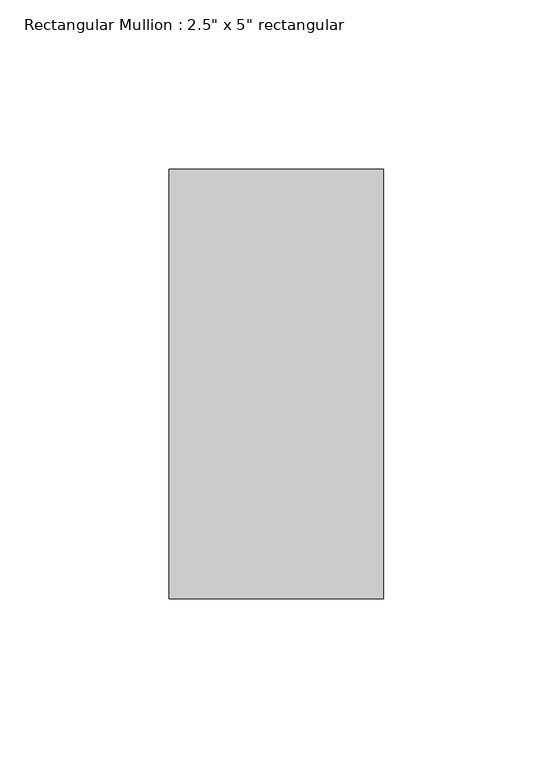
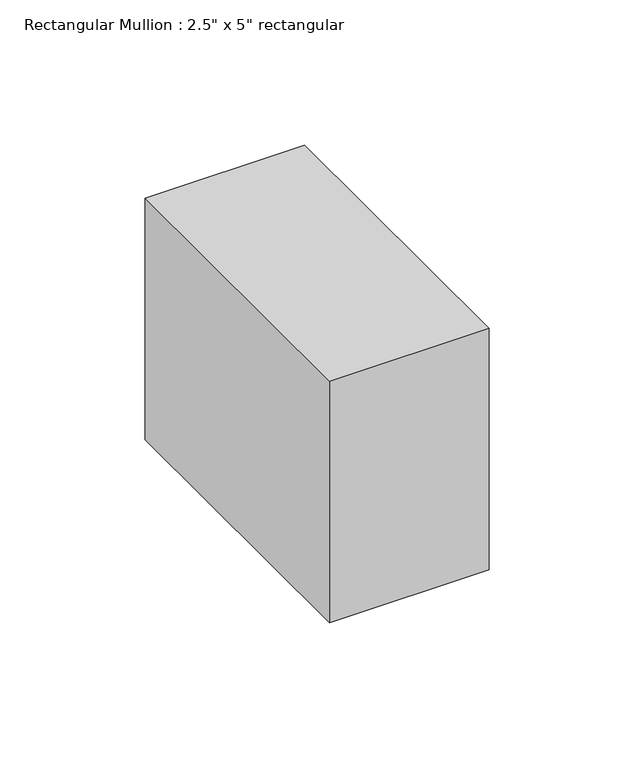
"""IFC4 building model written with IfcOpenShell, lengths in millimetres: member geometry."""

from ifc_helpers import new_model, si_unit, frame, origin, place, context, project, spatial, polyline, outline, extrude, source, transform, mapped, element, save


def member_5e78fce7(model_context):
    return source(origin(), model_context, "Body", "SweptSolid", [
        extrude(outline(polyline([(31.75, 63.5), (31.75, -63.5), (-31.75, -63.5), (-31.75, 63.5), (31.75, 63.5)])), frame((0.0, 0.0, -101.5332841), z_axis=(0.0, 0.0, 1.0), x_axis=(1.0, 0.0, 0.0)), (0.0, 0.0, 1.0), 101.5332841),
    ])


if __name__ == "__main__":
    model = new_model("IFC4")
    model_context = context("Model", 3, world=origin())
    ifc_project = project(units=[si_unit("LENGTHUNIT", "METRE", prefix="MILLI")], contexts=[model_context])
    site = spatial("IfcSite", under=ifc_project)
    building = spatial("IfcBuilding", under=site)
    placement = place(None, origin())
    member_shape = member_5e78fce7(model_context)
    element("IfcMember", 1, ObjectType="Rectangular Mullion : 2.5\" x 5\" rectangular", at=placement, inside=building, context=model_context, shape_type="MappedRepresentation", body=[
        mapped(member_shape, transform((0.0, 0.0, 0.0), x_axis=(1.0, 0.0, 0.0), y_axis=(0.0, 1.0, 0.0), z_axis=(0.0, 0.0, 1.0))),
    ])
    save(model, "model.ifc")

# Revit data of these elements
# Type "Rectangular Mullion : 2.5\" x 5\" rectangular"
#   built-in parameter 1007304 = 0.416667 (stored number, unit not read)
#   built-in parameter 1007301 = 0.104167 (stored number, unit not read)
#   built-in parameter 1007300 = 0.104167 (stored number, unit not read)
# Element 1 (IfcMember, "Rectangular Mullion : 2.5\" x 5\" rectangular")
#   Materials on its faces: "Aluminum"
# Materials
#   "Aluminum": class "Metal", colour RGB 247 247 247, transparency 0, Description = "Aluminum 6061", Cost = 0
